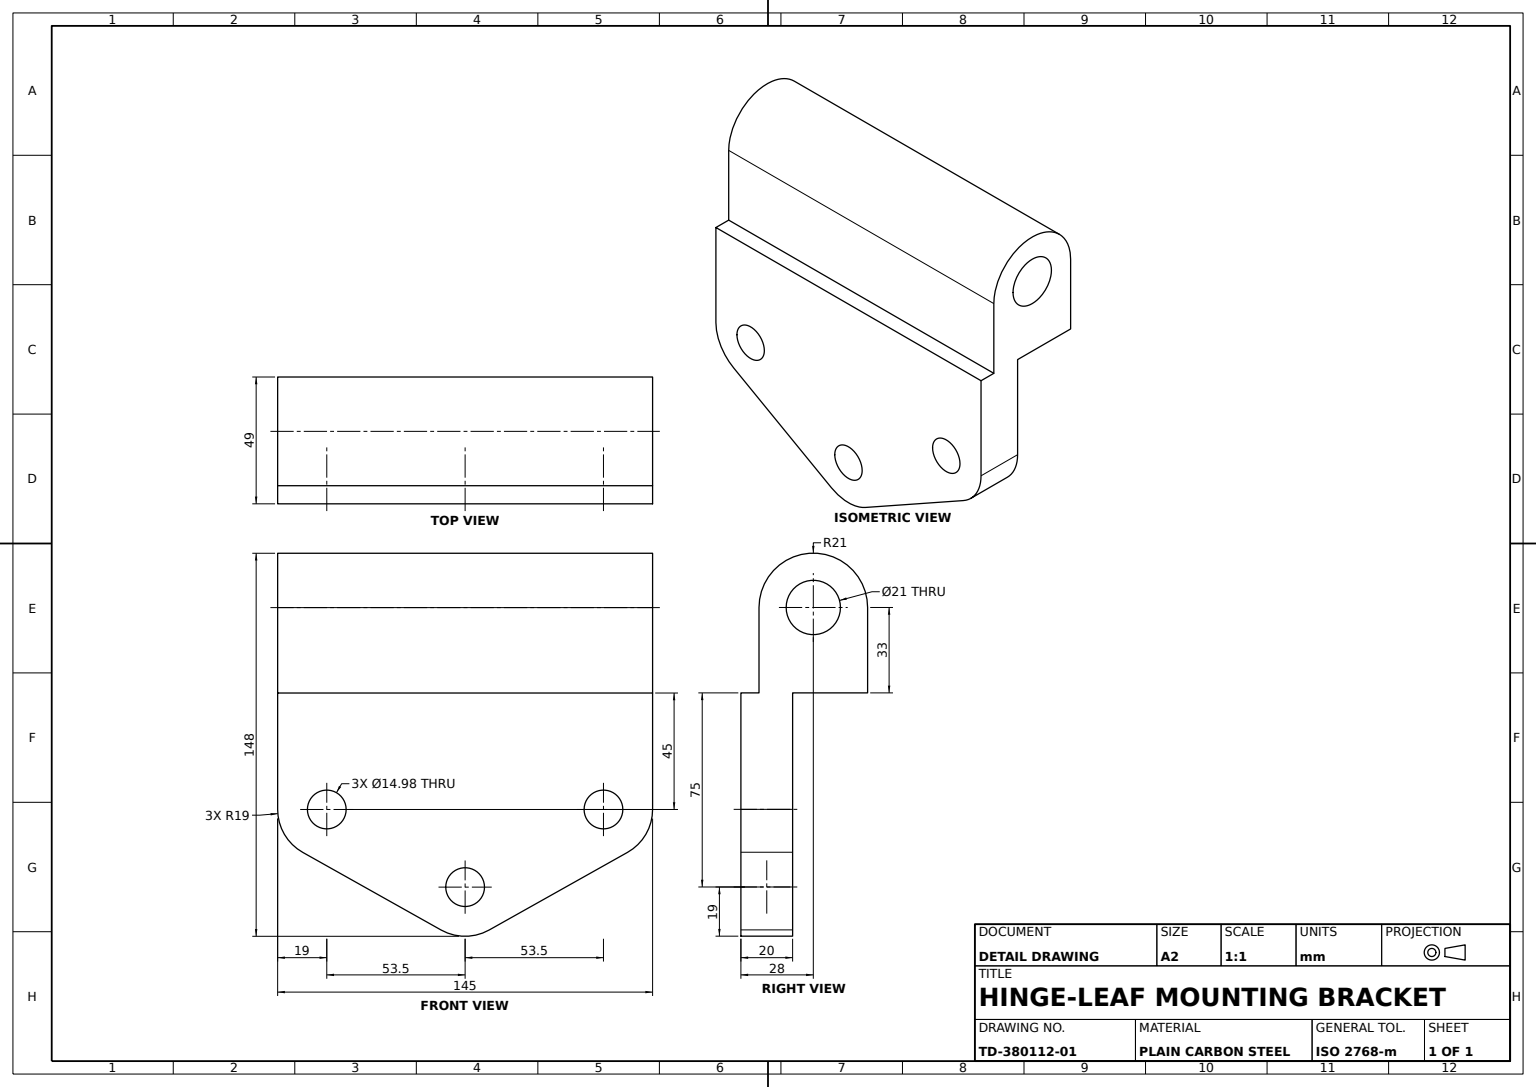
SolidWorks part; units mm, degrees
material "Plain Carbon Steel"
ref_plane "Front Plane" through (0, 0, 0) normal (0, 0, 1) x (1, 0, 0)
ref_plane "Top Plane" through (0, 0, 0) normal (0, 1, 0) x (1, 0, 0)
ref_plane "Right Plane" through (0, 0, 0) normal (1, 0, 0) x (0, 0, -1)
sketch "Base Plate Profile" plane through (0, 0, 0) normal (0, 0, 1) x (1, 0, 0)
  line L0 (0, 89.5541) -> (0, -113.978) construction
  line L1 (-72.5, 28.0645) -> (72.5, 28.0645)
  line L2 (-72.5, 28.0645) -> (-72.5, -16.9355)
  line L4 (72.5, 28.0645) -> (72.5, -16.9355)
  line L7 (-62.7929, -33.5078) -> (-9.2929, -63.5078)
  line L8 (62.7929, -33.5078) -> (9.2929, -63.5078)
  circle A0 centre (0, -46.9355) radius 7.4923
  circle A1 centre (53.5, -16.9355) radius 7.4923
  circle A2 centre (-53.5, -16.9355) radius 7.4923
  arc A3 (-9.2929, -63.5078) -> (9.2929, -63.5078) centre (0, -46.9355) ccw
  arc A4 (62.7929, -33.5078) -> (72.5, -16.9355) centre (53.5, -16.9355) ccw
  arc A5 (-72.5, -16.9355) -> (-62.7929, -33.5078) centre (-53.5, -16.9355) ccw
  point P0 (0, 0)
  dimension "D3" = 14.9845
  dimension "D4" = 38
  dimension "D5" = 19
  dimension "D1" = 145
  dimension "D2" = 28.0645
  dimension "D6" = 75
  dimension "D7" = 45
extrude "Base Plate 20mm" add sketch "Base Plate Profile" along normal blind 20
sketch "Hinge Knuckle Profile" plane through (0, 0, 0) normal (1, 0, 0) x (0, 0, -1)
  line L0 (8, 61.0645) -> (8, -4.9355) construction
  line L1 (29, 61.0645) -> (29, 28.0645)
  line L2 (-13, 61.0645) -> (-13, 28.0645)
  line L4 (-20, -16.9355) -> (-20, 28.0645) construction
  line L5 (-20, 28.0645) -> (0, 28.0645) construction
  line L6 (-13, 28.0645) -> (29, 28.0645)
  arc A0 (29, 61.0645) -> (-13, 61.0645) centre (8, 61.0645) ccw
  circle A2 centre (8, 61.0645) radius 10.5
  point P2 (8, 28.0645)
  dimension "D1" = 21
  dimension "D4" = 21
  dimension "D2" = 7
  dimension "D3" = 66
extrude "Hinge Knuckle 145mm" add sketch "Hinge Knuckle Profile" along normal mid plane 145
